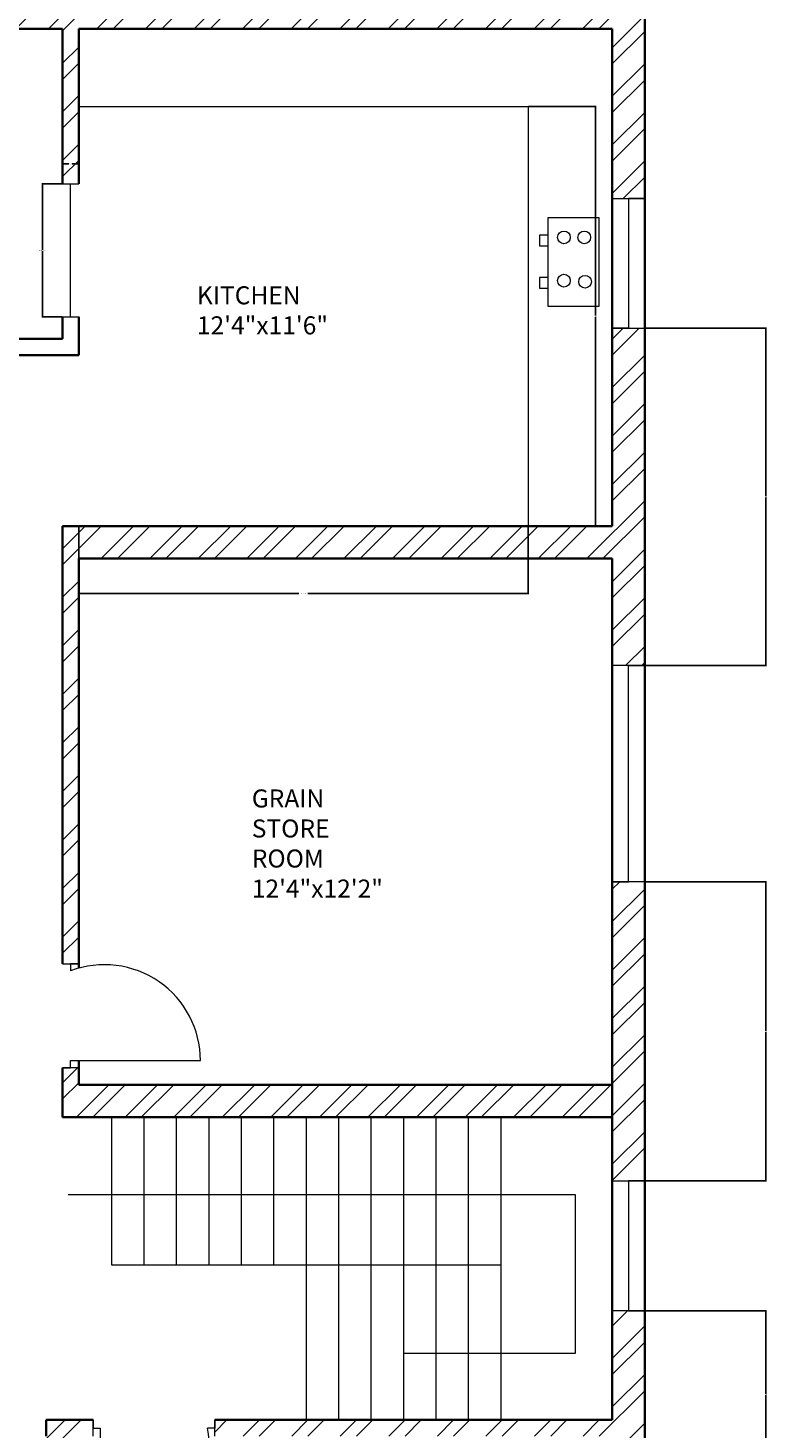
# Model space of a CAD drawing. Units: inches. Extents: x 1152 to 2588, y 1459 to 2618.
# Tile 6 of 17: x 1565 to 1770, y 1843 to 2231. Entities that reach past the tile are written whole.
import ezdxf

# ---------------------------------------------------------------- set-up
doc = ezdxf.new("R2010")
doc.units = ezdxf.units.IN
for name, color, linetype, lineweight in [('A-ANNO-DIMS', 2, 'Continuous', 18), ('A-AREA-IDEN', 7, 'Continuous', 18), ('A-DOOR', 4, 'Continuous', 18), ('A-EQPM', 9, 'Continuous', 18), ('A-FLOR-CASE', 30, 'Continuous', 18), ('A-FLOR-STRS', 3, 'Continuous', 18), ('A-GLAZ', 4, 'Continuous', 18), ('A-WALL', 7, 'Continuous', 35), ('A-WALL-PATT', 8, 'Continuous', 13)]:
    doc.layers.add(name, color=color, linetype=linetype, lineweight=lineweight)
doc.styles.get("Standard").update_dxf_attribs({"font": 'arial.ttf'})
doc.dimstyles.get("Standard").update_dxf_attribs({"dimtxt": 0.18, "dimasz": 0.18, "dimexe": 0.18, "dimexo": 0.0625, "dimgap": 0.09, "dimtad": 0, "dimtih": 1, "dimtoh": 1, "dimdec": 4, "dimzin": 0, "dimdsep": 46, "dimtxsty": 'Standard', "dimcen": 0.09, "dimadec": 0, "dimazin": 0, "dimtfac": 1, "dimtdec": 4, "dimtofl": 0, "dimtmove": 0, "dimatfit": 3, "dimfxl": 1, "dimtolj": 1, "dimtzin": 0, "dimarcsym": 0})

# ---------------------------------------------------------------- blocks, each defined once
blk = doc.blocks.new('DOOR-36-STORE')
for p, q in [((0, 28.88), (4.5, 28.88)), ((4.5, 28.88), (2.25, 28.88)), ((2.25, 28.88), (2.25, 26.88)), ((4.5, 0), (0, 0)), ((0, 0), (2.25, 0)), ((2.25, 0), (2.25, 2)), ((2.25, 2), (38.25, 2))]:
    blk.add_line(p, q)
blk.add_arc((11.65, 2), 26.6, 0, 110.707)
blk = doc.blocks.new('DOOR-36-HALL')
for p, q in [((0, 33.75), (0, 38.25)), ((0, 38.25), (0, 36)), ((0, 36), (2, 36)), ((2, 36), (2, 0)), ((33.77, 36), (31.77, 36)), ((33.77, 33.75), (33.77, 38.25)), ((33.77, 38.25), (33.77, 36))]:
    blk.add_line(p, q)
blk.add_arc((2, 30.31), 30.31, 270, 10.8162)
blk = doc.blocks.new('DOOR-STORE-OPENING')
for p, q in [((0, 36.9), (4.5, 36.9)), ((2.25, 0), (2.25, 36.9)), ((0, 0), (4.5, 0))]:
    blk.add_line(p, q)
blk = doc.blocks.new('WIN-60-EXT')
for p, q in [((0, 9), (0, 0)), ((60, 4.5), (60, 9)), ((60, 9), (60, 0)), ((0, 0), (0, 4.5)), ((0, 4.5), (60, 4.5))]:
    blk.add_line(p, q)
blk = doc.blocks.new('WIN-36')
for p, q in [((0, 36), (9, 36)), ((9, 36), (4.5, 36)), ((4.5, 36), (4.5, 0)), ((4.5, 0), (0, 0)), ((0, 0), (9, 0))]:
    blk.add_line(p, q)
blk = doc.blocks.new('WIN-36-STAIR')
for p, q in [((0, 36), (9, 36)), ((9, 36), (4.5, 36)), ((4.5, 36), (4.5, 0)), ((9, 0), (0, 0)), ((4.5, 0), (9, 0))]:
    blk.add_line(p, q)
blk = doc.blocks.new('STAIR-RETURN')
for p, q in [((12.04, 42.95), (12.04, 84)), ((21.04, 42.95), (21.04, 84)), ((30.04, 42.95), (30.04, 84)), ((39.04, 42.95), (39.04, 84)), ((48.04, 42.95), (48.04, 84)), ((57.04, 42.95), (57.04, 84)), ((66.04, 0), (66.04, 84)), ((75.04, 0), (75.04, 84)), ((84.04, 0), (84.04, 84)), ((93.04, 0), (93.04, 84)), ((102.04, 0), (102.04, 84)), ((111.04, 0), (111.04, 84)), ((120.04, 0), (120.04, 84)), ((0, 62.54), (140.6, 62.54)), ((140.6, 62.54), (140.6, 18.44)), ((120.04, 42.95), (12.04, 42.95)), ((140.6, 18.44), (93.04, 18.44))]:
    blk.add_line(p, q)
blk = doc.blocks.new('COUNTER-KITCHEN-L')
for p, q in [((0, 116.5), (124.66, 116.5)), ((124.66, 116.5), (124.66, 0))]:
    blk.add_line(p, q)
blk = doc.blocks.new('*D52')
at = {"layer": 'A-ANNO-DIMS', "color": 0, "lineweight": -2, "transparency": 16777216}
for p, q in [((1574.85, 2188.05), (1569.2, 2188.05)), ((1569.38, 2187.87), (1569.38, 2169.78)), ((1569.38, 2151.33), (1569.38, 2169.41)), ((1574.85, 2151.15), (1569.2, 2151.15))]:
    blk.add_line(p, q, dxfattribs=at)
at = {"layer": 'A-ANNO-DIMS', "color": 0, "transparency": 16777216}
for points in [[(1569.35, 2187.87), (1569.41, 2187.87), (1569.38, 2188.05)], [(1569.35, 2151.33), (1569.41, 2151.33), (1569.38, 2151.15)]]:
    blk.add_solid(points, dxfattribs=at)
at = {"layer": 'Defpoints', "color": 0, "transparency": 16777216}
for p in [(1569.38, 2188.05), (1574.92, 2188.05), (1574.92, 2151.15)]:
    blk.add_point(p, dxfattribs=at)
at = {"layer": 'A-ANNO-DIMS', "color": 0, "transparency": 16777216, "insert": (1569.38, 2169.6), "char_height": 0.18, "attachment_point": 5}
blk.add_mtext('\\A1;OPENING 37 TYP.', dxfattribs=at)
blk = doc.blocks.new('*D53')
at = {"layer": 'A-ANNO-DIMS', "color": 0, "lineweight": -2, "transparency": 16777216}
for p, q in [((1574.92, 2188.11), (1574.92, 2193.76)), ((1575.1, 2193.58), (1576.71, 2193.58)), ((1579.24, 2193.58), (1577.62, 2193.58)), ((1579.42, 2188.11), (1579.42, 2193.76))]:
    blk.add_line(p, q, dxfattribs=at)
at = {"layer": 'A-ANNO-DIMS', "color": 0, "transparency": 16777216}
for points in [[(1575.1, 2193.61), (1575.1, 2193.55), (1574.92, 2193.58)], [(1579.24, 2193.61), (1579.24, 2193.55), (1579.42, 2193.58)]]:
    blk.add_solid(points, dxfattribs=at)
at = {"layer": 'Defpoints', "color": 0, "transparency": 16777216}
for p in [(1579.42, 2193.58), (1574.92, 2188.05), (1579.42, 2188.05)]:
    blk.add_point(p, dxfattribs=at)
at = {"layer": 'A-ANNO-DIMS', "color": 0, "transparency": 16777216, "insert": (1577.17, 2193.58), "char_height": 0.18, "attachment_point": 5}
blk.add_mtext('\\A1;5 TYP.', dxfattribs=at)
blk = doc.blocks.new('*D68')
at = {"layer": 'A-ANNO-DIMS', "color": 0, "lineweight": -2, "transparency": 16777216}
for p, q in [((1579.42, 2092.98), (1579.42, 2074.17)), ((1704.08, 2092.98), (1704.08, 2074.17)), ((1579.6, 2074.35), (1640.49, 2074.35)), ((1703.9, 2074.35), (1643, 2074.35))]:
    blk.add_line(p, q, dxfattribs=at)
at = {"layer": 'A-ANNO-DIMS', "color": 0, "transparency": 16777216}
for points in [[(1579.6, 2074.38), (1579.6, 2074.32), (1579.42, 2074.35)], [(1703.9, 2074.38), (1703.9, 2074.32), (1704.08, 2074.35)]]:
    blk.add_solid(points, dxfattribs=at)
at = {"layer": 'Defpoints', "color": 0, "transparency": 16777216}
for p in [(1579.42, 2093.05), (1704.08, 2093.05), (1704.08, 2074.35)]:
    blk.add_point(p, dxfattribs=at)
at = {"layer": 'A-ANNO-DIMS', "color": 0, "transparency": 16777216, "insert": (1641.75, 2074.35), "char_height": 0.18, "attachment_point": 5}
blk.add_mtext('\\A1;COUNTER 125 TYP.', dxfattribs=at)
blk = doc.blocks.new('*D69')
at = {"layer": 'A-ANNO-DIMS', "color": 0, "lineweight": -2, "transparency": 16777216}
for p, q in [((1704.14, 2209.55), (1722.96, 2209.55)), ((1722.78, 2209.37), (1722.78, 2151.48)), ((1722.78, 2093.23), (1722.78, 2151.12)), ((1704.14, 2093.05), (1722.96, 2093.05))]:
    blk.add_line(p, q, dxfattribs=at)
at = {"layer": 'A-ANNO-DIMS', "color": 0, "transparency": 16777216}
for points in [[(1722.75, 2209.37), (1722.81, 2209.37), (1722.78, 2209.55)], [(1722.75, 2093.23), (1722.81, 2093.23), (1722.78, 2093.05)]]:
    blk.add_solid(points, dxfattribs=at)
at = {"layer": 'Defpoints', "color": 0, "transparency": 16777216}
for p in [(1704.08, 2209.55), (1722.78, 2209.55), (1704.08, 2093.05)]:
    blk.add_point(p, dxfattribs=at)
at = {"layer": 'A-ANNO-DIMS', "color": 0, "transparency": 16777216, "insert": (1722.78, 2151.3), "char_height": 0.18, "attachment_point": 5}
blk.add_mtext('\\A1;117 TYP.', dxfattribs=at)
blk = doc.blocks.new('*D74')
at = {"layer": 'A-ANNO-DIMS', "color": 0, "lineweight": -2, "transparency": 16777216}
for p, q in [((1736.48, 1875.36), (1770.2, 1875.36)), ((1770.02, 1875.18), (1770.02, 1852.24)), ((1770.02, 1828.94), (1770.02, 1851.88)), ((1736.48, 1828.76), (1770.2, 1828.76))]:
    blk.add_line(p, q, dxfattribs=at)
at = {"layer": 'A-ANNO-DIMS', "color": 0, "transparency": 16777216}
for points in [[(1769.99, 1875.18), (1770.05, 1875.18), (1770.02, 1875.36)], [(1769.99, 1828.94), (1770.05, 1828.94), (1770.02, 1828.76)]]:
    blk.add_solid(points, dxfattribs=at)
at = {"layer": 'Defpoints', "color": 0, "transparency": 16777216}
for p in [(1736.42, 1875.36), (1770.02, 1875.36), (1736.42, 1828.76)]:
    blk.add_point(p, dxfattribs=at)
at = {"layer": 'A-ANNO-DIMS', "color": 0, "transparency": 16777216, "insert": (1770.02, 1852.06), "char_height": 0.18, "attachment_point": 5}
blk.add_mtext('\\A1;46.59', dxfattribs=at)
blk = doc.blocks.new('*D75')
at = {"layer": 'A-ANNO-DIMS', "color": 0, "lineweight": -2, "transparency": 16777216}
for p, q in [((1736.48, 1994.38), (1770.2, 1994.38)), ((1770.02, 1994.2), (1770.02, 1953.05)), ((1770.02, 1911.54), (1770.02, 1952.69)), ((1736.48, 1911.36), (1770.2, 1911.36))]:
    blk.add_line(p, q, dxfattribs=at)
at = {"layer": 'A-ANNO-DIMS', "color": 0, "transparency": 16777216}
for points in [[(1769.99, 1994.2), (1770.05, 1994.2), (1770.02, 1994.38)], [(1769.99, 1911.54), (1770.05, 1911.54), (1770.02, 1911.36)]]:
    blk.add_solid(points, dxfattribs=at)
at = {"layer": 'Defpoints', "color": 0, "transparency": 16777216}
for p in [(1736.42, 1994.38), (1770.02, 1994.38), (1736.42, 1911.36)]:
    blk.add_point(p, dxfattribs=at)
at = {"layer": 'A-ANNO-DIMS', "color": 0, "transparency": 16777216, "insert": (1770.02, 1952.87), "char_height": 0.18, "attachment_point": 5}
blk.add_mtext('\\A1;83.03', dxfattribs=at)
blk = doc.blocks.new('*D76')
at = {"layer": 'A-ANNO-DIMS', "color": 0, "lineweight": -2, "transparency": 16777216}
for p, q in [((1736.48, 2147.97), (1770.2, 2147.97)), ((1770.02, 2147.79), (1770.02, 2101.36)), ((1770.02, 2054.56), (1770.02, 2101)), ((1736.48, 2054.38), (1770.2, 2054.38))]:
    blk.add_line(p, q, dxfattribs=at)
at = {"layer": 'A-ANNO-DIMS', "color": 0, "transparency": 16777216}
for points in [[(1769.99, 2147.79), (1770.05, 2147.79), (1770.02, 2147.97)], [(1769.99, 2054.56), (1770.05, 2054.56), (1770.02, 2054.38)]]:
    blk.add_solid(points, dxfattribs=at)
at = {"layer": 'Defpoints', "color": 0, "transparency": 16777216}
for p in [(1736.42, 2147.97), (1770.02, 2147.97), (1736.42, 2054.38)]:
    blk.add_point(p, dxfattribs=at)
at = {"layer": 'A-ANNO-DIMS', "color": 0, "transparency": 16777216, "insert": (1770.02, 2101.18), "char_height": 0.18, "attachment_point": 5}
blk.add_mtext('\\A1;93.59', dxfattribs=at)

msp = doc.modelspace()

# ---------------------------------------------------------------- hatches: boundary and pattern name
at = {"layer": 'A-WALL-PATT'}
h = msp.add_hatch(dxfattribs=at)
h.set_pattern_fill('ANSI32', color=256)
h.paths.add_polyline_path([(1408.9272, 2240.0458), (1276.4165, 2240.0458), (1276.4165, 2192.7491), (1285.4165, 2192.7491), (1285.4165, 2231.0458), (1369.4165, 2231.0458), (1369.4165, 2084.0458), (1526.9165, 2084.0458), (1526.9165, 2096.3728), (1524.6665, 2096.3728), (1522.4165, 2096.3728), (1522.4165, 2093.0458), (1378.4165, 2093.0458), (1378.4165, 2231.0458), (1408.9272, 2231.0458)])
h.paths.add_polyline_path([(1736.4165, 2240.0458), (1468.9272, 2240.0458), (1468.9272, 2231.0458), (1522.4165, 2231.0458), (1522.4165, 2127.3313), (1526.9165, 2127.3313), (1526.9165, 2231.0458), (1574.9165, 2231.0458), (1574.9165, 2188.0458), (1579.4165, 2188.0458), (1579.4165, 2231.0458), (1727.4165, 2231.0458), (1727.4165, 2183.9728), (1736.4165, 2183.9728)])
h.paths.add_polyline_path([(1285.4165, 2156.7491), (1276.4165, 2156.7491), (1276.4165, 2084.0458), (1285.4165, 2084.0458)], flags=17)
h.paths.add_polyline_path([(1285.4165, 2043.5458), (1445.4165, 2043.5458), (1445.4165, 1943.6503), (1454.4165, 1943.6503), (1454.4165, 2048.0458), (1276.4165, 2048.0458), (1276.4165, 2019.2077), (1280.9165, 2019.2077), (1285.4165, 2019.2077)])
h.paths.add_polyline_path([(1285.4165, 1959.2077), (1276.4165, 1959.2077), (1276.4165, 1891.1319), (1280.9165, 1891.1319), (1285.4165, 1891.1319), (1285.4165, 1901.0458), (1376.8505, 1901.0458), (1376.8505, 1903.2958), (1376.8505, 1905.5458), (1285.4165, 1905.5458)])
h.paths.add_polyline_path([(1518.4165, 1905.5458), (1399.2832, 1905.5458), (1399.2832, 1903.2958), (1399.2832, 1901.0458), (1405.4165, 1901.0458), (1405.4165, 1884.8579), (1409.9165, 1884.8579), (1409.9165, 1901.0458), (1513.9165, 1901.0458), (1513.9165, 1869.1706), (1518.4165, 1869.1706)])
h.paths.add_polyline_path([(1520.5229, 1845.0458), (1518.4165, 1845.0458), (1518.4165, 1849.2927), (1516.1665, 1849.2927), (1513.9165, 1849.2927), (1513.9165, 1845.0458), (1409.9165, 1845.0458), (1409.9165, 1860.8579), (1405.4165, 1860.8579), (1405.4165, 1845.0458), (1285.4165, 1845.0458), (1285.4165, 1867.1319), (1276.4165, 1867.1319), (1276.4165, 1635.0458), (1285.4165, 1635.0458), (1285.4165, 1836.0458), (1405.4165, 1836.0458), (1405.4165, 1635.0458), (1414.4165, 1635.0458), (1424.7277, 1635.0458), (1424.7277, 1639.5458), (1424.7277, 1644.0458), (1414.4165, 1644.0458), (1414.4165, 1836.0458), (1414.4165, 1840.5831), (1520.5229, 1840.5831)])
h.paths.add_polyline_path([(1579.4165, 1840.5458), (1583.4035, 1840.5458), (1583.4035, 1845.0458), (1579.4165, 1845.0458), (1570.4165, 1845.0458), (1570.4165, 1840.5831), (1570.4165, 1644.0458), (1548.2359, 1644.0458), (1548.2359, 1635.0458), (1611.2801, 1635.0458), (1611.2801, 1639.5458), (1611.2801, 1644.0458), (1579.4165, 1644.0458)])
h.paths.add_polyline_path([(1488.2359, 1644.0458), (1472.0663, 1644.0458), (1472.0663, 1635.0458), (1488.2359, 1635.0458), (1488.2359, 1639.5458)], flags=17)
h.paths.add_polyline_path([(1736.4165, 1701.1863), (1727.4165, 1701.1863), (1727.4165, 1644.0458), (1671.2801, 1644.0458), (1671.2801, 1635.0458), (1736.4165, 1635.0458)])
h.paths.add_polyline_path([(1736.4165, 2147.9728), (1727.4165, 2147.9728), (1727.4165, 2093.0458), (1579.4165, 2093.0458), (1574.9165, 2093.0458), (1574.9165, 1971.6501), (1579.4165, 1971.6501), (1579.4165, 2084.0458), (1727.4165, 2084.0458), (1727.4165, 2054.3847), (1736.4165, 2054.3847)])
h.paths.add_polyline_path([(1736.4165, 1994.3847), (1727.4165, 1994.3847), (1727.4165, 1911.3562), (1736.4165, 1911.3562)])
h.paths.add_polyline_path([(1736.4165, 1875.3562), (1727.4165, 1875.3562), (1727.4165, 1845.0458), (1617.1767, 1845.0458), (1617.1767, 1842.7958), (1617.1767, 1840.5458), (1618.9165, 1840.5458), (1618.9165, 1788.5458), (1618.9165, 1784.0458), (1627.8699, 1784.0458), (1627.8699, 1788.5458), (1623.4165, 1788.5458), (1623.4165, 1840.5458), (1727.4165, 1840.5458), (1727.4165, 1828.7619), (1736.4165, 1828.7619)])
h.paths.add_polyline_path([(1727.4165, 1938.0458), (1579.4165, 1938.0458), (1579.4165, 1942.7722), (1574.9165, 1942.7722), (1574.9165, 1929.0458), (1727.4165, 1929.0458)])

# ---------------------------------------------------------------- linework, layer by layer
at = {"layer": 'A-EQPM'}
for points in [[(1709.6436, 2178.7216), (1723.6997, 2178.7216), (1723.6997, 2154.0607), (1709.6436, 2154.0607)], [(1709.6436, 2173.8159), (1707.241, 2173.8159), (1707.241, 2170.8701), (1709.6436, 2170.8701)], [(1709.6436, 2162.061), (1707.241, 2162.061), (1707.241, 2159.1153), (1709.6436, 2159.1153)]]:
    msp.add_lwpolyline(points, close=True, dxfattribs=at)
for centre in [(1714.0047, 2173.1986), (1719.6457, 2173.1986), (1714.0047, 2161.1913), (1719.8643, 2160.8836)]:
    msp.add_circle(centre, 1.7674, dxfattribs=at)
at = {"layer": 'A-WALL'}
for p, q in [((1736.4165, 2240.0458), (1736.4165, 1635.0458)), ((1526.9165, 2231.0458), (1574.9165, 2231.0458)), ((1574.9165, 2231.0458), (1574.9165, 2188.0458)), ((1579.4165, 2231.0458), (1579.4165, 2188.0458)), ((1579.4165, 2231.0458), (1727.4165, 2231.0458)), ((1727.4165, 2231.0458), (1727.4165, 2093.0458)), ((1574.9165, 2151.1471), (1574.9165, 2145.0458)), ((1579.4165, 2151.1471), (1579.4165, 2140.5458)), ((1526.9165, 2145.0458), (1574.9165, 2145.0458)), ((1526.9165, 2140.5458), (1574.9165, 2140.5458)), ((1574.9165, 2140.5458), (1579.4165, 2140.5458)), ((1579.4165, 2093.0458), (1574.9165, 2093.0458)), ((1574.9165, 2093.0458), (1574.9165, 1971.6501)), ((1579.4165, 2093.0458), (1727.4165, 2093.0458)), ((1579.4165, 2084.0458), (1727.4165, 2084.0458)), ((1579.4165, 2084.0458), (1579.4165, 1970.3879)), ((1727.4165, 2084.0458), (1727.4165, 1845.0458)), ((1574.9165, 1942.7722), (1574.9165, 1929.0458)), ((1579.4165, 1944.7722), (1579.4165, 1938.0458)), ((1579.4165, 1938.0458), (1727.4165, 1938.0458)), ((1574.9165, 1929.0458), (1727.4165, 1929.0458)), ((1570.4165, 1840.5831), (1570.4165, 1845.0458)), ((1570.4165, 1845.0458), (1579.4165, 1845.0458)), ((1579.4165, 1845.0458), (1583.4035, 1845.0458)), ((1617.1767, 1845.0458), (1727.4165, 1845.0458))]:
    msp.add_line(p, q, dxfattribs=at)

# ---------------------------------------------------------------- block references
at = {"layer": 'A-DOOR'}
for name, p in [('DOOR-STORE-OPENING', (1574.917, 2151.147)), ('DOOR-36-STORE', (1574.917, 1942.772)), ('DOOR-36-HALL', (1583.404, 1806.796))]:
    msp.add_blockref(name, p, dxfattribs=at)
at = {"layer": 'A-FLOR-CASE'}
msp.add_blockref('COUNTER-KITCHEN-L', (1579.417, 2093.046), dxfattribs=at)
at = {"layer": 'A-FLOR-STRS'}
msp.add_blockref('STAIR-RETURN', (1576.524, 1845.046), dxfattribs=at)
at = {"layer": 'A-GLAZ'}
for name, p in [('WIN-36', (1727.417, 2147.9727)), ('WIN-36-STAIR', (1727.417, 1875.356))]:
    msp.add_blockref(name, p, dxfattribs=at)
at = {"layer": 'A-GLAZ', "extrusion": (0, 0, -1), "zscale": -1, "rotation": 90}
msp.add_blockref('WIN-60-EXT', (-1727.4167, 1994.3846), dxfattribs=at)

# ---------------------------------------------------------------- texts
at = {"layer": 'A-AREA-IDEN', "char_height": 5, "attachment_point": 1}
for s, width, insert in [('KITCHEN\\P12\'4"x11\'6"', 152.387291, (1612.1949, 2159.6206)), ('GRAIN\\PSTORE\\PROOM\\P12\'4"x12\'2"', 141.12584, (1627.4218, 2020.0056))]:
    msp.add_mtext_dynamic_manual_height_columns(s, width=width, gutter_width=12.5, heights=[0], dxfattribs=dict(at, insert=insert))

# ---------------------------------------------------------------- dimensions: what is measured, and where the dimension line sits
at = {"layer": 'A-ANNO-DIMS'}
for base, p1, p2, text, picture, middle in [((1722.7759214108, 2209.5458348558), (1704.0768708813, 2093.0458348558), (1704.0768708813, 2209.5458348558), '<> TYP.', '*D69', (1722.7759214108, 2151.2958348558)), ((1569.3817, 2188.0458), (1574.9165, 2151.1471), (1574.9165, 2188.0458), 'OPENING <> TYP.', '*D52', (1569.3817, 2169.5964))]:
    dim = msp.add_linear_dim(base=base, p1=p1, p2=p2, angle=90, text=text, dimstyle='Standard', override={"dimdec": 0, "dimlfac": 1, "dimrnd": 0, "dimzin": 0, "dimdsep": 46, "dimlunit": 2}, dxfattribs=at)
    dim.commit()
    dim.dimension.update_dxf_attribs({"geometry": picture, "text_midpoint": middle})
for base, p1, p2, text, picture, middle in [((1579.4165340182, 2193.5806515744), (1574.9165340182, 2188.0458348558), (1579.4165340182, 2188.0458348558), '<> TYP.', '*D53', (1577.1665340182, 2193.5806515744)), ((1704.0769, 2074.3468), (1579.4165, 2093.0458), (1704.0769, 2093.0458), 'COUNTER <> TYP.', '*D68', (1641.7467, 2074.3468))]:
    dim = msp.add_linear_dim(base=base, p1=p1, p2=p2, text=text, dimstyle='Standard', override={"dimdec": 0, "dimlfac": 1, "dimrnd": 0, "dimzin": 0, "dimdsep": 46, "dimlunit": 2}, dxfattribs=at)
    dim.commit()
    dim.dimension.update_dxf_attribs({"geometry": picture, "text_midpoint": middle})
for base, p1, p2, picture, middle in [((1770.0165, 2147.9728), (1736.4165, 2054.3847), (1736.4165, 2147.9728), '*D76', (1770.0165, 2101.1788)), ((1770.0165, 1994.3847), (1736.4165, 1911.3562), (1736.4165, 1994.3847), '*D75', (1770.0165, 1952.8705)), ((1770.0165, 1875.3562), (1736.4165, 1828.7619), (1736.4165, 1875.3562), '*D74', (1770.0165, 1852.0591))]:
    dim = msp.add_linear_dim(base=base, p1=p1, p2=p2, angle=90, dimstyle='Standard', override={"dimdec": 2, "dimlfac": 1, "dimrnd": 0, "dimzin": 0, "dimdsep": 46, "dimlunit": 2}, dxfattribs=at)
    dim.commit()
    dim.dimension.update_dxf_attribs({"geometry": picture, "text_midpoint": middle})

doc.saveas('drawing.dxf')
